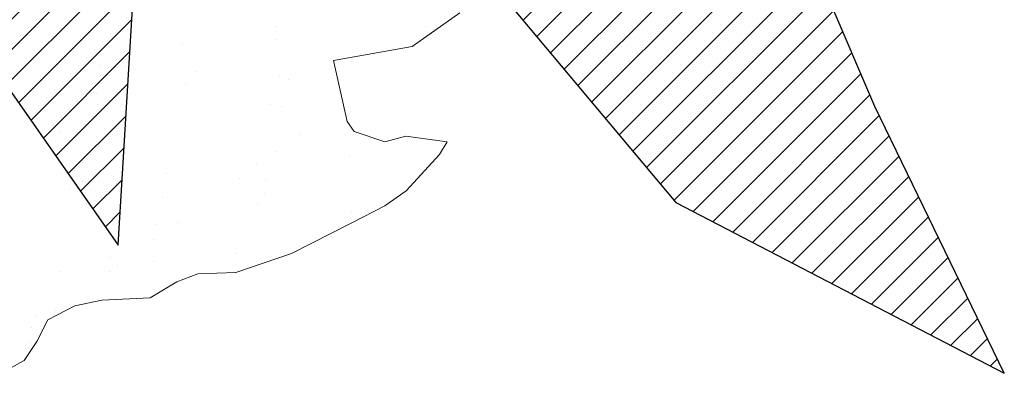
# Model space of a CAD drawing. Units: inches. Extents: x 1986 to 21484, y -1816 to 2016.
# Tile 53 of 85: x 3671.752 to 3678.86, y 1868.178 to 1870.798. Entities that reach past the tile are written whole.
import ezdxf

# ---------------------------------------------------------------- set-up
doc = ezdxf.new("R2010")
doc.units = ezdxf.units.IN
doc.layers.add('L-PLNT', color=84, linetype='Continuous', lineweight=13)
doc.layers.add('vfolhas', color=114, linetype='Continuous', lineweight=5)
doc.layers.add('vfolha2', color=110, linetype='Continuous')
doc.layers.add('vfolhas2', color=102, linetype='Continuous')
pattern_1 = [(45, (-2446.5133113, 50.986076), (-0.004419417382, 0.004419417382), [])]

# ---------------------------------------------------------------- blocks, each defined once
blk = doc.blocks.new('arbusto_PB_verde_grande')
at = {"layer": 'vfolha2'}
h = blk.add_hatch(dxfattribs=at)
h.set_pattern_fill('ANSI31', color=256, scale=0.05, style=0)
h.set_pattern_definition(pattern_1)
h.paths.add_polyline_path([(-0.18963, 0.29704), (-0.08553, 0.20192), (-0.10785, 0.25007), (-0.13202, 0.31865), (-0.25096, 0.48479), (-0.44952, 0.5505), (-0.37946, 0.43789)])
h.paths.add_polyline_path([(0.07911, -0.4071), (0.08214, -0.50631), (0.17255, -0.6355), (0.18428, -0.44151), (0.14904, -0.29177), (0.02625, -0.03934), (0.03527, -0.25376)])
at = {"layer": 'vfolhas'}
h = blk.add_hatch(dxfattribs=at)
h.set_pattern_fill('ANSI31', color=256, scale=0.05, style=0)
h.set_pattern_definition(pattern_1)
h.paths.add_polyline_path([(0.33611, -0.623), (0.43251, -0.67306), (0.39456, -0.59485), (0.3303, -0.44464), (0.29522, -0.42585), (0.15794, -0.31007), (0.14904, -0.29177), (0.18428, -0.44151)])
at = {"layer": 'vfolha2'}
for p, q in [((0.17255, -0.6355), (0.18428, -0.44151)), ((0.08214, -0.50631), (0.17255, -0.6355))]:
    blk.add_line(p, q, dxfattribs=at)
at = {"layer": 'vfolhas2'}
for p, q in [((0.18428, -0.44151), (0.33611, -0.623)), ((0.39456, -0.59485), (0.32904, -0.4417)), ((0.43251, -0.67306), (0.39456, -0.59485)), ((0.33611, -0.623), (0.43251, -0.67306))]:
    blk.add_line(p, q, dxfattribs=at)
blk = doc.blocks.new('PLANT-SHRUB')
for p, q in [((2169.4208, 1904.2347), (2169.7765, 1904.2605)), ((2169.7765, 1904.2605), (2169.9621, 1904.2347)), ((2169.3177, 1904.2038), (2169.4208, 1904.2347)), ((2169.508, 1903.9698), (2169.3177, 1904.2038)), ((2169.9621, 1904.2347), (2170.225, 1904.1574)), ((2170.225, 1904.1574), (2170.6889, 1904.0235)), ((2170.1677, 1904.0968), (2170.1677, 1904.0968)), ((2170.6889, 1904.0235), (2171.0756, 1903.8484)), ((2169.6474, 1903.8965), (2169.508, 1903.9698)), ((2169.7574, 1903.6913), (2169.6474, 1903.8965)), ((2171.0756, 1903.8484), (2171.2818, 1903.6681)), ((2169.8971, 1903.7934), (2169.8971, 1903.7934)), ((2169.7427, 1903.6034), (2169.7574, 1903.6913)), ((2170.9766, 1903.7545), (2170.9766, 1903.7545)), ((2171.2818, 1903.6681), (2171.4313, 1903.6063)), ((2168.6132, 1903.5887), (2169.0313, 1903.5301)), ((2169.5154, 1903.215), (2169.7427, 1903.6034)), ((2170.5359, 1903.5707), (2170.5359, 1903.5707)), ((2170.6202, 1903.5899), (2170.6202, 1903.5899)), ((2171.4313, 1903.6063), (2171.6529, 1903.5599)), ((2171.6529, 1903.5599), (2171.9179, 1903.3329)), ((2168.863, 1903.4895), (2168.863, 1903.4895)), ((2169.0313, 1903.5301), (2169.5154, 1903.215)), ((2170.4623, 1903.5032), (2170.4623, 1903.5032)), ((2170.06, 1903.4393), (2170.06, 1903.4393)), ((2170.2681, 1903.4119), (2170.2681, 1903.4119)), ((2170.4362, 1903.3797), (2170.4362, 1903.3797)), ((2170.593, 1903.3691), (2170.593, 1903.3691)), ((2171.4585, 1903.3846), (2171.4585, 1903.3846)), ((2171.9179, 1903.3329), (2172.088, 1903.2298)), ((2171.1359, 1903.2977), (2171.1359, 1903.2977)), ((2171.3439, 1903.2703), (2171.3439, 1903.2703)), ((2172.4643, 1903.2298), (2172.6241, 1903.2659)), ((2172.6241, 1903.2659), (2172.9437, 1903.1835)), ((2169.5154, 1903.215), (2169.5154, 1903.215)), ((2170.0135, 1903.2033), (2170.0135, 1903.2033)), ((2171.2581, 1903.2011), (2171.2581, 1903.2011)), ((2171.6688, 1903.2275), (2171.6688, 1903.2275)), ((2171.7374, 1903.22), (2171.7374, 1903.22)), ((2172.088, 1903.2298), (2172.2993, 1903.168)), ((2172.2993, 1903.168), (2172.4643, 1903.2298)), ((2172.5027, 1903.1988), (2172.5027, 1903.1988)), ((2170.0645, 1903.1387), (2170.0645, 1903.1387)), ((2171.6637, 1903.1525), (2171.6637, 1903.1525)), ((2172.2117, 1903.156), (2172.2117, 1903.156)), ((2172.4197, 1903.1287), (2172.4197, 1903.1287)), ((2169.8449, 1903.096), (2169.8449, 1903.096)), ((2171.0895, 1903.0937), (2171.0895, 1903.0937)), ((2172.3342, 1903.0915), (2172.3342, 1903.0915)), ((2169.8719, 1903.0233), (2169.8719, 1903.0233)), ((2170.9514, 1902.9844), (2170.9514, 1902.9844)), ((2171.9976, 1902.971), (2171.9976, 1902.971)), ((2169.7168, 1902.8201), (2169.7168, 1902.8201)), ((2171.2659, 1902.7879), (2171.2659, 1902.7879)), ((2169.6431, 1902.7526), (2169.6431, 1902.7526)), ((2170.2974, 1902.5891), (2170.2974, 1902.5891)), ((2170.411, 1902.6096), (2170.411, 1902.6096)), ((2171.4334, 1902.6145), (2171.4334, 1902.6145)), ((2171.542, 1902.5868), (2171.542, 1902.5868)), ((2170.9182, 1902.4693), (2170.9182, 1902.4693)), ((2170.2245, 1902.3829), (2170.2245, 1902.3829)), ((2170.8445, 1902.4018), (2170.8445, 1902.4018)), ((2170.7674, 1902.3114), (2170.7674, 1902.3114)), ((2170.9754, 1902.284), (2170.9754, 1902.284)), ((2170.9262, 1902.2143), (2170.9262, 1902.2143)), ((2170.9353, 1902.2003), (2170.9353, 1902.2003)), ((2171.3003, 1902.2412), (2171.3003, 1902.2412)), ((2170.7668, 1902.0929), (2170.7668, 1902.0929)), ((2170.4467, 1902.0373), (2170.4467, 1902.0373))]:
    blk.add_line(p, q)

msp = doc.modelspace()

# ---------------------------------------------------------------- block references
at = {"layer": 'L-PLNT', "rotation": 223.1883365522388}
msp.add_blockref('PLANT-SHRUB', (3953.27, 4742.9646), dxfattribs=at)
at = {"layer": 'L-PLNT', "xscale": 24.60366729364114, "yscale": 24.60366729364114, "zscale": 24.60366729364114}
msp.add_blockref('arbusto_PB_verde_grande', (3668.2184, 1884.8051), dxfattribs=at)

doc.saveas('drawing.dxf')
